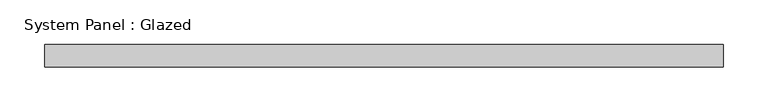
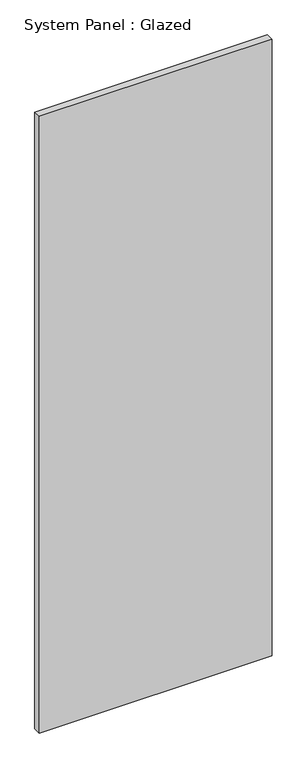
"""IFC4 building model written with IfcOpenShell, lengths in millimetres: plate geometry, System Panel : Glazed."""

from ifc_helpers import new_model, si_unit, origin, origin_with_axes, place, context, project, spatial, polyline, outline, extrude, source, transform, mapped, element, save


def system_panel_glazed_13fc6ba1(model_context):
    return source(origin(), model_context, "Body", "SweptSolid", [
        extrude(outline(polyline([(381.0, 19.05), (-381.0, 19.05), (-381.0, 44.45), (381.0, 44.45), (381.0, 19.05)])), origin_with_axes(), (0.0, 0.0, 1.0), 2133.6),
    ])


if __name__ == "__main__":
    model = new_model("IFC4")
    model_context = context("Model", 3, world=origin())
    ifc_project = project(units=[si_unit("LENGTHUNIT", "METRE", prefix="MILLI")], contexts=[model_context])
    site = spatial("IfcSite", under=ifc_project)
    building = spatial("IfcBuilding", under=site)
    placement = place(None, origin())
    system_panel_glazed_shape = system_panel_glazed_13fc6ba1(model_context)
    element("IfcPlate", 1, ObjectType="System Panel : Glazed", at=placement, inside=building, context=model_context, shape_type="MappedRepresentation", body=[
        mapped(system_panel_glazed_shape, transform((0.0, 0.0, 0.0), x_axis=(1.0, 0.0, 0.0), y_axis=(0.0, 1.0, 0.0), z_axis=(0.0, 0.0, 1.0))),
    ])
    save(model, "model.ifc")

# Revit data of these elements
# Type "System Panel : Glazed"
#   Construction Type Id = "GSP4R"
#   Analytic Construction = "1/8 in Pilkington single glazing"
#   Visual Light Transmittance = 0.9
#   Solar Heat Gain Coefficient = 0.86
#   Heat Transfer Coefficient (U) = 1.18115 BTU/(h·ft²·°F)
#   Define Thermal Properties by = 1
# Element 1 (IfcPlate, "System Panel : Glazed")
#   Materials on its faces: "Glass"
# Materials
#   "Glass": class "Glass", colour RGB 0 128 192, transparency 0.75, Description = "Soda Lime Glass", Cost = 0
